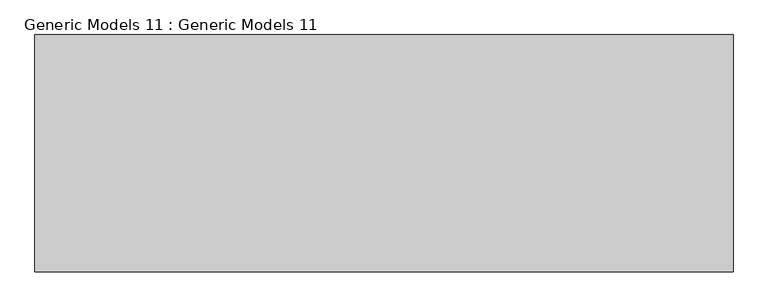
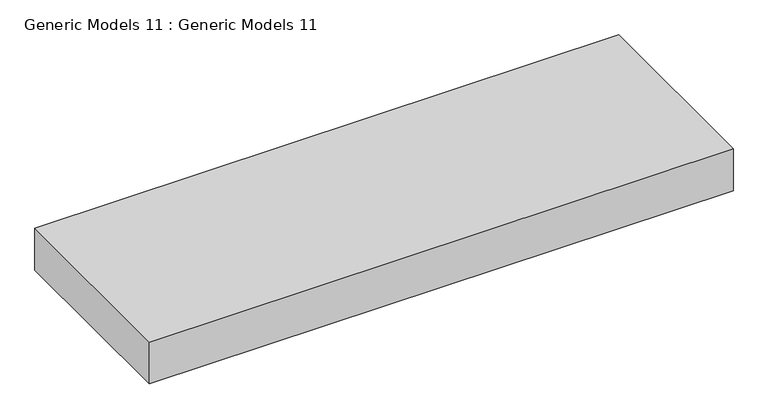
"""IFC4 building model written with IfcOpenShell, lengths in millimetres: proxy geometry, Generic Models 11 : Generic Models 11."""

from ifc_helpers import new_model, si_unit, frame, origin, place, context, project, spatial, polyline, outline, extrude, source, transform, mapped, element, save


def generic_models_11_generic_models_11_3010cca1(model_context):
    return source(origin(), model_context, "Body", "SweptSolid", [
        extrude(outline(polyline([(6327.3005956, -12972.6972423), (1273.3423568, -12972.6972423), (1273.3423568, -11254.0073314), (6327.3005956, -11254.0073314), (6327.3005956, -12972.6972423)])), frame((0.0, 0.0, 3200.4), z_axis=(0.0, 0.0, 1.0), x_axis=(1.0, 0.0, 0.0)), (0.0, 0.0, 1.0), 384.175),
    ])


if __name__ == "__main__":
    model = new_model("IFC4")
    model_context = context("Model", 3, world=origin())
    ifc_project = project(units=[si_unit("LENGTHUNIT", "METRE", prefix="MILLI")], contexts=[model_context])
    site = spatial("IfcSite", under=ifc_project)
    building = spatial("IfcBuilding", under=site)
    placement = place(None, origin())
    generic_models_11_generic_models_11_shape = generic_models_11_generic_models_11_3010cca1(model_context)
    element("IfcBuildingElementProxy", 1, Name="Generic Models 11 : Generic Models 11", ObjectType="Generic Models 11 : Generic Models 11", at=placement, inside=building, context=model_context, shape_type="MappedRepresentation", body=[
        mapped(generic_models_11_generic_models_11_shape, transform((0.0, 0.0, 0.0), x_axis=(1.0, 0.0, 0.0), y_axis=(0.0, 1.0, 0.0), z_axis=(0.0, 0.0, 1.0))),
    ])
    save(model, "model.ifc")

# Revit data of these elements
# Element 1 (IfcBuildingElementProxy, "Generic Models 11 : Generic Models 11")
#   Materials on its faces: "Clad - White"
# Materials
#   "Clad - White": class "Wood", colour RGB 242 242 238, transparency 0, Cost = 0
